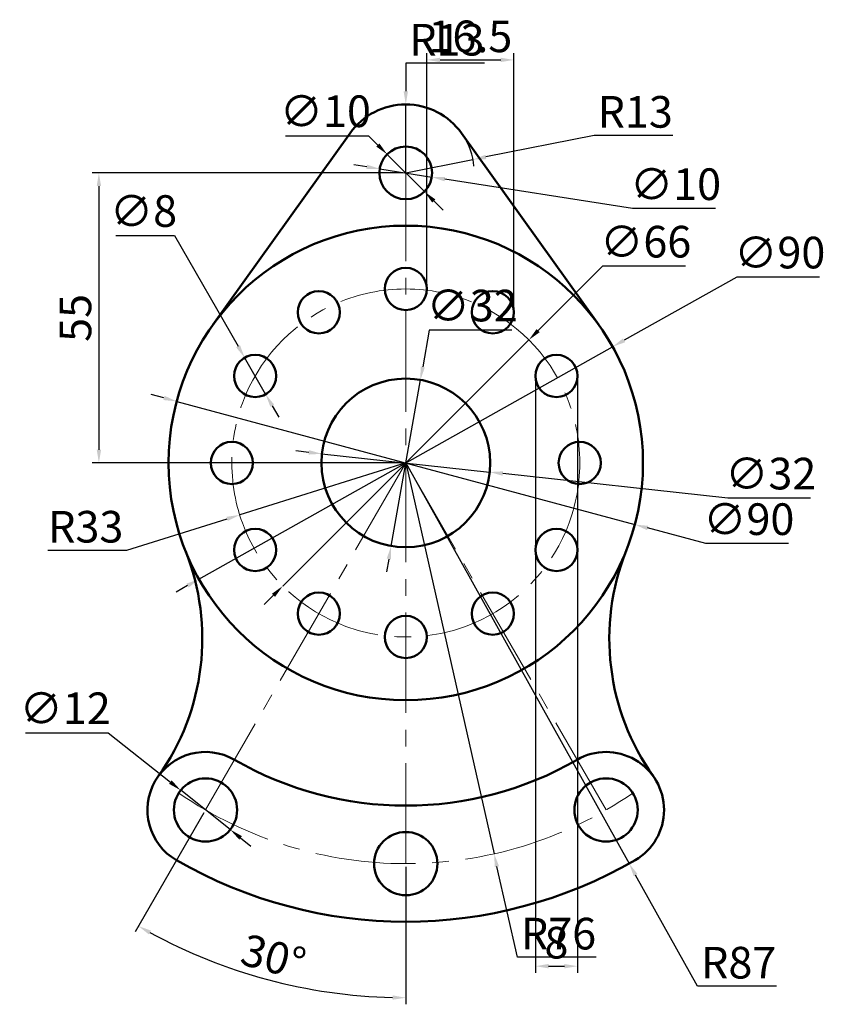
# Model space of a CAD drawing. Units: millimetres. Extents: x 15 to 167, y 24 to 211.
import ezdxf

# ---------------------------------------------------------------- set-up
doc = ezdxf.new("R2010")
doc.units = ezdxf.units.MM
doc.linetypes.add('CENTER2', pattern=[28.575, 19.05, -3.175, 3.175, -3.175])
for name, color, linetype, lineweight in [('M-CNTR', 4, 'CENTER2', 18), ('M-DIMS', 2, 'Continuous', 25), ('M-OUTL', 7, 'Continuous', 50)]:
    doc.layers.add(name, color=color, linetype=linetype, lineweight=lineweight)
doc.styles.get("Standard").update_dxf_attribs({"font": 'arial.ttf'})
doc.dimstyles.new('ISO-25', dxfattribs={"dimtxt": 6, "dimasz": 2.5, "dimexe": 1.25, "dimexo": 0.625, "dimtad": 1, "dimtoh": 1, "dimdec": 0, "dimtxsty": 'Standard', "dimcen": 2.5, "dimadec": 0, "dimazin": 0, "dimtfac": 1, "dimtdec": 0, "dimtmove": 0, "dimatfit": 3, "dimfxl": 1, "dimarcsym": 0})

# ---------------------------------------------------------------- blocks, each defined once
blk = doc.blocks.new('*U1')
blk.add_circle((0, 0), 4)
blk = doc.blocks.new('*U2')
at = {"layer": 'M-OUTL', "color": 0, "linetype": 'ByBlock', "lineweight": -2, "transparency": 16777216}
blk.add_blockref('*U1', (87.78, 159.7), dxfattribs=at)
for p, rotation in [((71.28, 155.28), 30.00000000000002), ((104.28, 155.28), 330.0000000000001), ((59.2, 143.2), 60.00000000000003), ((116.36, 143.2), 300), ((54.78, 126.7), 90.00000000000006), ((120.78, 126.7), 270), ((59.2, 110.2), 120), ((116.36, 110.2), 240), ((71.28, 98.12), 150), ((104.28, 98.12), 210), ((87.78, 93.7), 180)]:
    blk.add_blockref('*U1', p, dxfattribs=dict(at, rotation=rotation))
blk = doc.blocks.new('*D3')
at = {"layer": 'Defpoints', "color": 0, "transparency": 16777216}
for p in [(100.53, 184.24), (87.78, 181.7)]:
    blk.add_point(p, dxfattribs=at)
at = {"layer": 'M-DIMS', "color": 0, "lineweight": -2, "transparency": 16777216}
for p, q in [((123.5, 188.82), (102.98, 184.73)), ((138.47, 188.82), (123.5, 188.82)), ((87.78, 181.7), (100.53, 184.24))]:
    blk.add_line(p, q, dxfattribs=at)
blk.add_arc((87.78, 181.7), 13, 5.7614, 32.8239, dxfattribs=at)
at = {"layer": 'M-DIMS', "color": 0, "transparency": 16777216}
blk.add_solid([(102.9, 185.14), (103.06, 184.32), (100.53, 184.24)], dxfattribs=at)
at = {"layer": 'M-DIMS', "color": 0, "transparency": 16777216, "insert": (131.3, 192.51), "char_height": 6, "attachment_point": 5}
blk.add_mtext('R13', dxfattribs=at)
blk = doc.blocks.new('*D4')
at = {"layer": 'Defpoints', "color": 0, "transparency": 16777216}
for p in [(82.84, 182.47), (92.72, 180.92)]:
    blk.add_point(p, dxfattribs=at)
at = {"layer": 'M-DIMS', "color": 0, "lineweight": -2, "transparency": 16777216}
for p, q in [((80.37, 182.86), (77.9, 183.25)), ((82.84, 182.47), (92.72, 180.92)), ((130.78, 174.94), (95.19, 180.53)), ((146.51, 174.94), (130.78, 174.94))]:
    blk.add_line(p, q, dxfattribs=at)
at = {"layer": 'M-DIMS', "color": 0, "transparency": 16777216}
for points in [[(80.44, 183.27), (80.31, 182.45), (82.84, 182.47)], [(95.25, 180.94), (95.12, 180.12), (92.72, 180.92)]]:
    blk.add_solid(points, dxfattribs=at)
at = {"layer": 'M-DIMS', "color": 0, "transparency": 16777216, "insert": (138.96, 178.79), "char_height": 6, "attachment_point": 5}
blk.add_mtext('∅10', dxfattribs=at)
blk = doc.blocks.new('*D5')
at = {"layer": 'Defpoints', "color": 0, "transparency": 16777216}
for p in [(87.78, 181.7), (29.56, 126.7), (87.78, 126.7)]:
    blk.add_point(p, dxfattribs=at)
at = {"layer": 'M-DIMS', "color": 0, "lineweight": -2, "transparency": 16777216}
for p, q in [((87.16, 181.7), (28.31, 181.7)), ((29.56, 179.2), (29.56, 129.2)), ((87.16, 126.7), (28.31, 126.7))]:
    blk.add_line(p, q, dxfattribs=at)
at = {"layer": 'M-DIMS', "color": 0, "transparency": 16777216}
for points in [[(29.15, 179.2), (29.98, 179.2), (29.56, 181.7)], [(29.15, 129.2), (29.98, 129.2), (29.56, 126.7)]]:
    blk.add_solid(points, dxfattribs=at)
at = {"layer": 'M-DIMS', "color": 0, "transparency": 16777216, "insert": (25.89, 154.2), "char_height": 6, "attachment_point": 5, "rotation": 90}
blk.add_mtext('55', dxfattribs=at)
blk = doc.blocks.new('*D6')
at = {"layer": 'Defpoints', "color": 0, "transparency": 16777216}
for p in [(57.21, 146.67), (61.19, 139.73)]:
    blk.add_point(p, dxfattribs=at)
at = {"layer": 'M-DIMS', "color": 0, "lineweight": -2, "transparency": 16777216}
for p, q in [((32.8, 169.84), (43.9, 169.84)), ((43.9, 169.84), (55.96, 148.83)), ((61.19, 139.73), (57.21, 146.67)), ((62.44, 137.56), (63.68, 135.39))]:
    blk.add_line(p, q, dxfattribs=at)
at = {"layer": 'M-DIMS', "color": 0, "transparency": 16777216}
for points in [[(56.33, 149.04), (55.6, 148.63), (57.21, 146.67)], [(62.8, 137.77), (62.08, 137.35), (61.19, 139.73)]]:
    blk.add_solid(points, dxfattribs=at)
at = {"layer": 'M-DIMS', "color": 0, "transparency": 16777216, "insert": (38.03, 173.7), "char_height": 6, "attachment_point": 5}
blk.add_mtext('∅8', dxfattribs=at)
blk = doc.blocks.new('*D7')
at = {"layer": 'Defpoints', "color": 0, "transparency": 16777216}
for p in [(71.87, 128.43), (103.69, 124.97)]:
    blk.add_point(p, dxfattribs=at)
at = {"layer": 'M-DIMS', "color": 0, "lineweight": -2, "transparency": 16777216}
for p, q in [((69.39, 128.7), (66.9, 128.97)), ((71.87, 128.43), (103.69, 124.97)), ((148.86, 120.05), (106.17, 124.7)), ((164.55, 120.05), (148.86, 120.05))]:
    blk.add_line(p, q, dxfattribs=at)
at = {"layer": 'M-DIMS', "color": 0, "transparency": 16777216}
for points in [[(69.43, 129.12), (69.34, 128.29), (71.87, 128.43)], [(106.22, 125.11), (106.13, 124.28), (103.69, 124.97)]]:
    blk.add_solid(points, dxfattribs=at)
at = {"layer": 'M-DIMS', "color": 0, "transparency": 16777216, "insert": (157.02, 123.9), "char_height": 6, "attachment_point": 5}
blk.add_mtext('∅32', dxfattribs=at)
blk = doc.blocks.new('*D8')
at = {"layer": 'Defpoints', "color": 0, "transparency": 16777216}
for p in [(87.78, 126.7), (56.29, 116.84)]:
    blk.add_point(p, dxfattribs=at)
at = {"layer": 'M-DIMS', "color": 0, "lineweight": -2, "transparency": 16777216}
for p, q in [((87.78, 126.7), (56.29, 116.84)), ((34.85, 110.13), (53.9, 116.09)), ((19.89, 110.13), (34.85, 110.13))]:
    blk.add_line(p, q, dxfattribs=at)
at = {"layer": 'M-DIMS', "color": 0, "transparency": 16777216}
blk.add_solid([(53.78, 116.49), (54.03, 115.7), (56.29, 116.84)], dxfattribs=at)
at = {"layer": 'M-DIMS', "color": 0, "transparency": 16777216, "insert": (27.06, 113.82), "char_height": 6, "attachment_point": 5}
blk.add_mtext('R33', dxfattribs=at)
blk = doc.blocks.new('*D9')
at = {"layer": 'Defpoints', "color": 0, "transparency": 16777216}
for p in [(45.08, 64.61), (54.48, 57.15)]:
    blk.add_point(p, dxfattribs=at)
at = {"layer": 'M-DIMS', "color": 0, "lineweight": -2, "transparency": 16777216}
for p, q in [((15.64, 75.54), (31.33, 75.54)), ((31.33, 75.54), (43.12, 66.17)), ((54.48, 57.15), (45.08, 64.61)), ((56.44, 55.59), (58.39, 54.04))]:
    blk.add_line(p, q, dxfattribs=at)
at = {"layer": 'M-DIMS', "color": 0, "transparency": 16777216}
for points in [[(43.38, 66.49), (42.87, 65.84), (45.08, 64.61)], [(56.7, 55.92), (56.18, 55.27), (54.48, 57.15)]]:
    blk.add_solid(points, dxfattribs=at)
at = {"layer": 'M-DIMS', "color": 0, "transparency": 16777216, "insert": (23.17, 79.39), "char_height": 6, "attachment_point": 5}
blk.add_mtext('∅12', dxfattribs=at)
blk = doc.blocks.new('*D10')
at = {"layer": 'Defpoints', "color": 0, "transparency": 16777216}
for p in [(44.32, 138.38), (131.24, 115.01)]:
    blk.add_point(p, dxfattribs=at)
at = {"layer": 'M-DIMS', "color": 0, "lineweight": -2, "transparency": 16777216}
for p, q in [((41.91, 139.03), (39.5, 139.68)), ((44.32, 138.38), (131.24, 115.01)), ((144.68, 111.4), (133.65, 114.37)), ((160.41, 111.4), (144.68, 111.4))]:
    blk.add_line(p, q, dxfattribs=at)
at = {"layer": 'M-DIMS', "color": 0, "transparency": 16777216}
for points in [[(42.02, 139.43), (41.8, 138.63), (44.32, 138.38)], [(133.76, 114.77), (133.54, 113.96), (131.24, 115.01)]]:
    blk.add_solid(points, dxfattribs=at)
at = {"layer": 'M-DIMS', "color": 0, "transparency": 16777216, "insert": (152.86, 115.26), "char_height": 6, "attachment_point": 5}
blk.add_mtext('∅90', dxfattribs=at)
blk = doc.blocks.new('*D11')
at = {"layer": 'Defpoints', "color": 0, "transparency": 16777216}
for p in [(87.78, 126.7), (104.53, 52.57)]:
    blk.add_point(p, dxfattribs=at)
at = {"layer": 'M-DIMS', "color": 0, "lineweight": -2, "transparency": 16777216}
for p, q in [((87.78, 126.7), (104.53, 52.57)), ((108.95, 32.96), (105.08, 50.13)), ((123.91, 32.96), (108.95, 32.96))]:
    blk.add_line(p, q, dxfattribs=at)
at = {"layer": 'M-DIMS', "color": 0, "transparency": 16777216}
blk.add_solid([(105.48, 50.22), (104.67, 50.04), (104.53, 52.57)], dxfattribs=at)
at = {"layer": 'M-DIMS', "color": 0, "transparency": 16777216, "insert": (116.75, 36.65), "char_height": 6, "attachment_point": 5}
blk.add_mtext('R76', dxfattribs=at)
blk = doc.blocks.new('*D12')
at = {"layer": 'Defpoints', "color": 0, "transparency": 16777216}
for p in [(87.78, 126.7), (130.16, 50.72)]:
    blk.add_point(p, dxfattribs=at)
at = {"layer": 'M-DIMS', "color": 0, "lineweight": -2, "transparency": 16777216}
for p, q in [((87.78, 126.7), (130.16, 50.72)), ((143.14, 27.45), (131.38, 48.53)), ((158.1, 27.45), (143.14, 27.45))]:
    blk.add_line(p, q, dxfattribs=at)
at = {"layer": 'M-DIMS', "color": 0, "transparency": 16777216}
blk.add_solid([(131.74, 48.74), (131.01, 48.33), (130.16, 50.72)], dxfattribs=at)
at = {"layer": 'M-DIMS', "color": 0, "transparency": 16777216, "insert": (150.93, 31.14), "char_height": 6, "attachment_point": 5}
blk.add_mtext('R87', dxfattribs=at)
blk = doc.blocks.new('*D13')
at = {"layer": 'Defpoints', "color": 0, "transparency": 16777216}
for p in [(87.78, 181.7), (87.78, 126.7), (49.78, 60.88), (87.78, 50.7), (53.09, 31.39)]:
    blk.add_point(p, dxfattribs=at)
at = {"layer": 'M-DIMS', "color": 0, "lineweight": -2, "transparency": 16777216}
for p, q in [((49.47, 60.34), (36.44, 37.78)), ((87.78, 50.07), (87.78, 24.02))]:
    blk.add_line(p, q, dxfattribs=at)
blk.add_arc((87.78, 126.7), 101.43, 241.4123, 268.5877, dxfattribs=at)
at = {"layer": 'M-DIMS', "color": 0, "transparency": 16777216}
for points in [[(39.04, 37.27), (39.45, 38), (37.07, 38.86)], [(85.29, 25.72), (85.28, 24.89), (87.78, 25.27)]]:
    blk.add_solid(points, dxfattribs=at)
at = {"layer": 'M-DIMS', "color": 0, "transparency": 16777216, "insert": (62.48, 32.29), "char_height": 6, "attachment_point": 5, "rotation": 345}
blk.add_mtext('30°', dxfattribs=at)
blk = doc.blocks.new('FLANGE-HOLE-D12')
blk.add_circle((6, 6), 6)
blk = doc.blocks.new('*D15')
at = {"layer": 'Defpoints', "color": 0, "transparency": 16777216}
for p in [(112.36, 143.2), (120.36, 143.2), (120.36, 31.25)]:
    blk.add_point(p, dxfattribs=at)
at = {"layer": 'M-DIMS', "color": 0, "lineweight": -2, "transparency": 16777216}
for p, q in [((112.36, 142.57), (112.36, 30)), ((120.36, 142.57), (120.36, 30)), ((114.86, 31.25), (117.86, 31.25))]:
    blk.add_line(p, q, dxfattribs=at)
at = {"layer": 'M-DIMS', "color": 0, "transparency": 16777216}
for points in [[(114.86, 31.67), (114.86, 30.84), (112.36, 31.25)], [(117.86, 31.67), (117.86, 30.84), (120.36, 31.25)]]:
    blk.add_solid(points, dxfattribs=at)
at = {"layer": 'M-DIMS', "color": 0, "transparency": 16777216, "insert": (116.36, 34.94), "char_height": 6, "attachment_point": 5}
blk.add_mtext('8', dxfattribs=at)
blk = doc.blocks.new('*D16')
at = {"layer": 'Defpoints', "color": 0, "transparency": 16777216}
for p in [(108.28, 203.14), (91.78, 159.7), (108.28, 155.28)]:
    blk.add_point(p, dxfattribs=at)
at = {"layer": 'M-DIMS', "color": 0, "lineweight": -2, "transparency": 16777216}
for p, q in [((91.78, 160.32), (91.78, 204.39)), ((108.28, 155.9), (108.28, 204.39)), ((94.28, 203.14), (105.78, 203.14))]:
    blk.add_line(p, q, dxfattribs=at)
at = {"layer": 'M-DIMS', "color": 0, "transparency": 16777216}
for points in [[(94.28, 203.56), (94.28, 202.73), (91.78, 203.14)], [(105.78, 203.56), (105.78, 202.73), (108.28, 203.14)]]:
    blk.add_solid(points, dxfattribs=at)
at = {"layer": 'M-DIMS', "color": 0, "transparency": 16777216, "insert": (100.03, 206.83), "char_height": 6, "attachment_point": 5}
blk.add_mtext('16.5', dxfattribs=at)
blk = doc.blocks.new('*D17')
at = {"layer": 'Defpoints', "color": 0, "transparency": 16777216}
for p in [(90.56, 142.45), (85, 110.94)]:
    blk.add_point(p, dxfattribs=at)
at = {"layer": 'M-DIMS', "color": 0, "lineweight": -2, "transparency": 16777216}
for p, q in [((92.23, 151.91), (90.99, 144.92)), ((107.91, 151.91), (92.23, 151.91)), ((85, 110.94), (90.56, 142.45)), ((84.57, 108.48), (84.13, 106.02))]:
    blk.add_line(p, q, dxfattribs=at)
at = {"layer": 'M-DIMS', "color": 0, "transparency": 16777216}
for points in [[(90.58, 144.99), (91.4, 144.84), (90.56, 142.45)], [(84.16, 108.55), (84.98, 108.41), (85, 110.94)]]:
    blk.add_solid(points, dxfattribs=at)
at = {"layer": 'M-DIMS', "color": 0, "transparency": 16777216, "insert": (100.38, 155.77), "char_height": 6, "attachment_point": 5}
blk.add_mtext('∅32', dxfattribs=at)
blk = doc.blocks.new('*D18')
at = {"layer": 'Defpoints', "color": 0, "transparency": 16777216}
for p in [(127.01, 148.74), (48.55, 104.66)]:
    blk.add_point(p, dxfattribs=at)
at = {"layer": 'M-DIMS', "color": 0, "lineweight": -2, "transparency": 16777216}
for p, q in [((150.55, 161.96), (129.19, 149.96)), ((166.28, 161.96), (150.55, 161.96)), ((48.55, 104.66), (127.01, 148.74)), ((46.37, 103.43), (44.19, 102.21))]:
    blk.add_line(p, q, dxfattribs=at)
at = {"layer": 'M-DIMS', "color": 0, "transparency": 16777216}
for points in [[(128.99, 150.32), (129.4, 149.6), (127.01, 148.74)], [(46.16, 103.8), (46.57, 103.07), (48.55, 104.66)]]:
    blk.add_solid(points, dxfattribs=at)
at = {"layer": 'M-DIMS', "color": 0, "transparency": 16777216, "insert": (158.73, 165.82), "char_height": 6, "attachment_point": 5}
blk.add_mtext('∅90', dxfattribs=at)
blk = doc.blocks.new('*D19')
at = {"layer": 'Defpoints', "color": 0, "transparency": 16777216}
for p in [(111.12, 150.03), (64.45, 103.36)]:
    blk.add_point(p, dxfattribs=at)
at = {"layer": 'M-DIMS', "color": 0, "lineweight": -2, "transparency": 16777216}
for p, q in [((125.12, 164.03), (112.88, 151.8)), ((140.86, 164.03), (125.12, 164.03)), ((64.45, 103.36), (111.12, 150.03)), ((62.68, 101.6), (60.91, 99.83))]:
    blk.add_line(p, q, dxfattribs=at)
at = {"layer": 'M-DIMS', "color": 0, "transparency": 16777216}
for points in [[(112.59, 152.09), (113.18, 151.5), (111.12, 150.03)], [(62.38, 101.89), (62.97, 101.3), (64.45, 103.36)]]:
    blk.add_solid(points, dxfattribs=at)
at = {"layer": 'M-DIMS', "color": 0, "transparency": 16777216, "insert": (133.3, 167.89), "char_height": 6, "attachment_point": 5}
blk.add_mtext('∅66', dxfattribs=at)
blk = doc.blocks.new('*D20')
at = {"layer": 'Defpoints', "color": 0, "transparency": 16777216}
for p in [(87.78, 194.7), (87.78, 181.7)]:
    blk.add_point(p, dxfattribs=at)
at = {"layer": 'M-DIMS', "color": 0, "lineweight": -2, "transparency": 16777216}
for p, q in [((102.74, 202.5), (87.78, 202.5)), ((87.78, 202.5), (87.78, 197.2)), ((87.78, 181.7), (87.78, 194.7))]:
    blk.add_line(p, q, dxfattribs=at)
at = {"layer": 'M-DIMS', "color": 0, "transparency": 16777216}
blk.add_solid([(87.36, 197.2), (88.2, 197.2), (87.78, 194.7)], dxfattribs=at)
at = {"layer": 'M-DIMS', "color": 0, "transparency": 16777216, "insert": (95.57, 206.19), "char_height": 6, "attachment_point": 5}
blk.add_mtext('R13', dxfattribs=at)
blk = doc.blocks.new('*D21')
at = {"layer": 'Defpoints', "color": 0, "transparency": 16777216}
for p in [(84.25, 185.23), (91.32, 178.16)]:
    blk.add_point(p, dxfattribs=at)
at = {"layer": 'M-DIMS', "color": 0, "lineweight": -2, "transparency": 16777216}
for p, q in [((64.98, 188.77), (80.71, 188.77)), ((80.71, 188.77), (82.48, 187)), ((91.32, 178.16), (84.25, 185.23)), ((93.08, 176.39), (94.85, 174.63))]:
    blk.add_line(p, q, dxfattribs=at)
at = {"layer": 'M-DIMS', "color": 0, "transparency": 16777216}
for points in [[(82.77, 187.3), (82.18, 186.71), (84.25, 185.23)], [(93.38, 176.69), (92.79, 176.1), (91.32, 178.16)]]:
    blk.add_solid(points, dxfattribs=at)
at = {"layer": 'M-DIMS', "color": 0, "transparency": 16777216, "insert": (72.53, 192.63), "char_height": 6, "attachment_point": 5}
blk.add_mtext('∅10', dxfattribs=at)

msp = doc.modelspace()

# ---------------------------------------------------------------- linework, layer by layer
at = {"layer": 'M-CNTR'}
msp.add_line((87.78, 50.7), (87.78, 181.7), dxfattribs=at)
msp.add_lwpolyline([(125.78, 60.88), (87.78, 126.7), (49.78, 60.88)], dxfattribs=at)
msp.add_circle((87.78, 126.7), 33, dxfattribs=at)
msp.add_arc((87.78, 126.7), 76, 235.4755, 304.5245, dxfattribs=at)
at = {"layer": 'M-OUTL'}
msp.add_lwpolyline([(51.18, 152.88), (77.21, 189.26, -0.514167), (98.35, 189.26), (124.38, 152.88)], format="xyb", dxfattribs=at)
msp.add_lwpolyline([(55.28, 70.41, 1), (44.28, 51.35, 0.267949), (131.28, 51.35, 1), (120.28, 70.41, -0.267949)], format="xyb", close=True, dxfattribs=at)
for centre, radius in [((87.78, 181.7), 5), ((87.78, 126.7), 45), ((87.78, 126.7), 16)]:
    msp.add_circle(centre, radius, dxfattribs=at)
for centre, start, end in [((4.18, 93.38), 324.526, 21.7288), ((171.39, 93.38), 158.2712, 215.474)]:
    msp.add_arc(centre, 45, start, end, dxfattribs=at)

# ---------------------------------------------------------------- block references
for name, p in [('*U2', (0, 0)), ('FLANGE-HOLE-D12', (43.78, 54.88)), ('FLANGE-HOLE-D12', (119.78, 54.88)), ('FLANGE-HOLE-D12', (81.78, 44.7))]:
    msp.add_blockref(name, p, dxfattribs=at)

# ---------------------------------------------------------------- dimensions: what is measured, and where the dimension line sits
at = {"layer": 'M-DIMS'}
for center, mpoint, override, picture, middle in [((87.78, 181.7), (87.78, 194.7), {"dimdec": 0, "dimlfac": 1, "dimrnd": 0, "dimzin": 0, "dimdsep": 46, "dimlunit": 2}, '*D20', (95.57, 202.5)), ((87.78, 181.7), (100.53, 184.24), {"dimclrd": 0, "dimclre": 0, "dimclrt": 0}, '*D3', (123.5, 188.82)), ((87.78, 126.7), (56.29, 116.84), {"dimclrd": 0, "dimclre": 0, "dimclrt": 0}, '*D8', (27.06, 110.13)), ((87.78, 126.7), (104.53, 52.57), {"dimclrd": 0, "dimclre": 0, "dimclrt": 0}, '*D11', (116.75, 32.96)), ((87.78, 126.7), (130.16, 50.72), {"dimclrd": 0, "dimclre": 0, "dimclrt": 0}, '*D12', (150.93, 27.45))]:
    dim = msp.add_radius_dim(center=center, mpoint=mpoint, dimstyle='ISO-25', override=override, dxfattribs=at)
    dim.commit()
    dim.dimension.update_dxf_attribs({"geometry": picture, "text_midpoint": middle, "dimtype": 164})
for base, p1, p2, override, picture, middle in [((108.28, 203.14), (91.78, 159.7), (108.28, 155.28), {"dimdec": 1, "dimlfac": 1, "dimrnd": 0, "dimzin": 0, "dimdsep": 46, "dimlunit": 2}, '*D16', (100.03, 206.83)), ((120.36, 31.25), (112.36, 143.2), (120.36, 143.2), {"dimdec": 0, "dimlfac": 1, "dimrnd": 0, "dimzin": 0, "dimdsep": 46, "dimlunit": 2}, '*D15', (116.36, 34.94))]:
    dim = msp.add_linear_dim(base=base, p1=p1, p2=p2, dimstyle='ISO-25', override=override, dxfattribs=at)
    dim.commit()
    dim.dimension.update_dxf_attribs({"geometry": picture, "text_midpoint": middle})
for p1, p2, override, picture, middle in [((91.32, 178.16), (84.25, 185.23), {"dimdec": 0, "dimlfac": 1, "dimrnd": 0, "dimzin": 0, "dimdsep": 46, "dimlunit": 2}, '*D21', (72.53, 188.77)), ((82.84, 182.47), (92.72, 180.92), {"dimclrd": 0, "dimclre": 0, "dimclrt": 0}, '*D4', (130.78, 174.94)), ((61.19, 139.73), (57.21, 146.67), {"dimclrd": 0, "dimclre": 0, "dimclrt": 0}, '*D6', (38.03, 169.84)), ((64.45, 103.36), (111.12, 150.03), {"dimdec": 0, "dimlfac": 1, "dimrnd": 0, "dimzin": 0, "dimdsep": 46, "dimlunit": 2}, '*D19', (133.3, 164.03)), ((48.55, 104.66), (127.01, 148.74), {"dimdec": 0, "dimlfac": 1, "dimrnd": 0, "dimzin": 0, "dimdsep": 46, "dimlunit": 2}, '*D18', (158.73, 161.96)), ((85, 110.94), (90.56, 142.45), {"dimdec": 0, "dimlfac": 1, "dimrnd": 0, "dimzin": 0, "dimdsep": 46, "dimlunit": 2}, '*D17', (100.38, 151.91)), ((44.32, 138.38), (131.24, 115.01), {"dimclrd": 0, "dimclre": 0, "dimclrt": 0}, '*D10', (152.86, 111.4)), ((71.87, 128.43), (103.69, 124.97), {"dimclrd": 0, "dimclre": 0, "dimclrt": 0}, '*D7', (148.86, 120.05)), ((54.48, 57.15), (45.08, 64.61), {"dimclrd": 0, "dimclre": 0, "dimclrt": 0}, '*D9', (23.17, 75.54))]:
    dim = msp.add_diameter_dim_2p(p1=p1, p2=p2, dimstyle='ISO-25', override=override, dxfattribs=at)
    dim.commit()
    dim.dimension.update_dxf_attribs({"geometry": picture, "text_midpoint": middle, "dimtype": 163})
dim = msp.add_linear_dim(base=(29.56, 126.7), p1=(87.78, 181.7), p2=(87.78, 126.7), angle=90, dimstyle='ISO-25', override={"dimclrd": 0, "dimclre": 0, "dimclrt": 0}, dxfattribs=at)
dim.commit()
dim.dimension.update_dxf_attribs({"geometry": '*D5', "text_midpoint": (25.89, 154.2)})
dim = msp.add_angular_dim_2l(base=(53.09, 31.39), line1=((87.78, 126.7), (49.78, 60.88)), line2=((87.78, 50.7), (87.78, 181.7)), dimstyle='ISO-25', override={"dimclrd": 0, "dimclre": 0, "dimclrt": 0}, dxfattribs=at)
dim.commit()
dim.dimension.update_dxf_attribs({"geometry": '*D13', "text_midpoint": (62.48, 32.29)})

doc.saveas('drawing.dxf')
